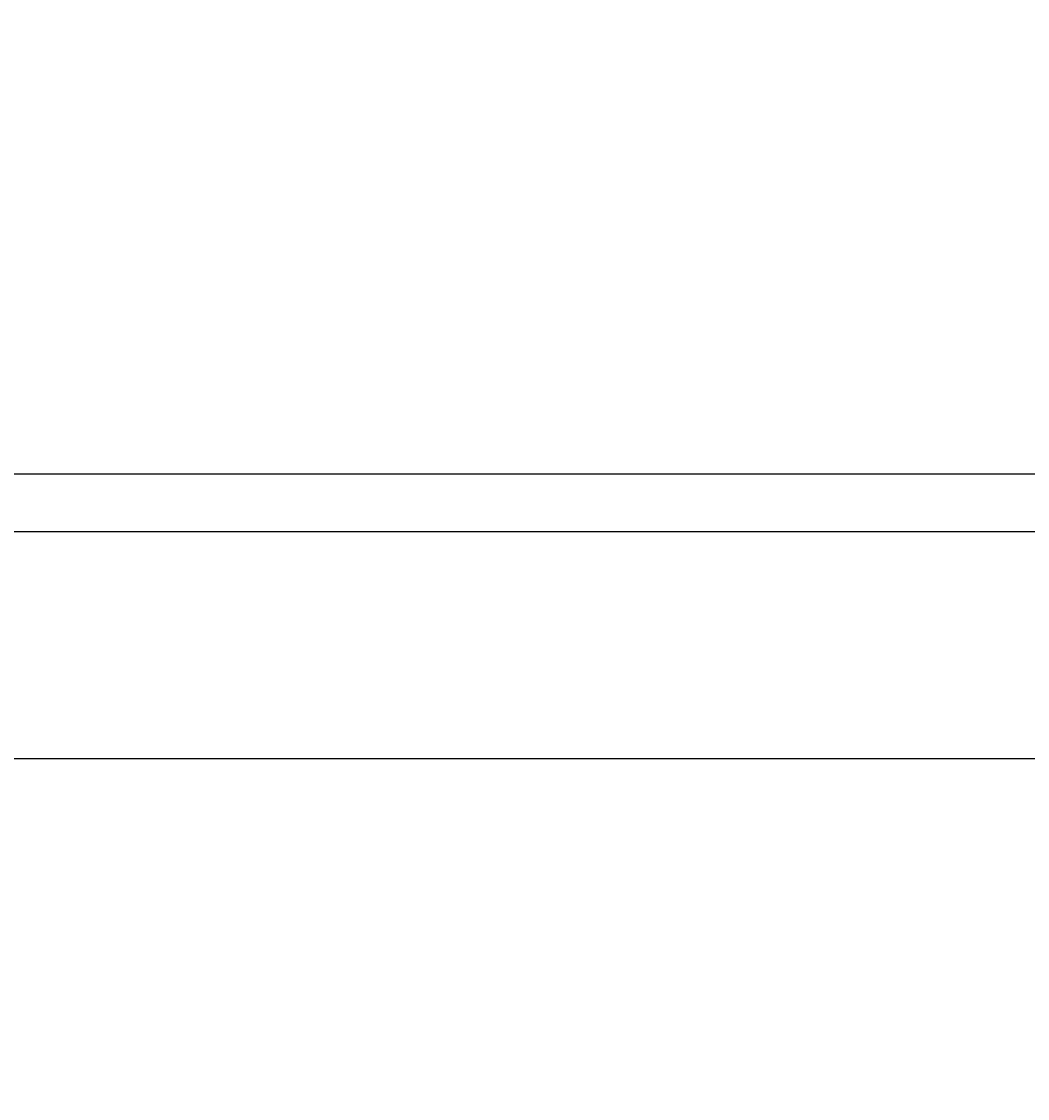
# Model space of a CAD drawing. Units: inches. Extents: x 1998 to 2588, y 1139 to 1977.
# Tile 96 of 134: x 2370 to 2397, y 1580 to 1608. Entities that reach past the tile are written whole.
import ezdxf

# ---------------------------------------------------------------- set-up
doc = ezdxf.new("R2010")
doc.units = ezdxf.units.IN
doc.layers.add('A-ANNO-DIMS', color=2, linetype='Continuous', lineweight=18)
doc.styles.get("Standard").update_dxf_attribs({"font": 'arial.ttf'})
doc.dimstyles.get("Standard").update_dxf_attribs({"dimtxt": 0.18, "dimasz": 0.18, "dimexe": 0.18, "dimexo": 0.0625, "dimgap": 0.09, "dimtad": 0, "dimtih": 1, "dimtoh": 1, "dimdec": 4, "dimzin": 0, "dimdsep": 46, "dimtxsty": 'Standard', "dimcen": 0.09, "dimadec": 0, "dimazin": 0, "dimtfac": 1, "dimtdec": 4, "dimtofl": 0, "dimtmove": 0, "dimatfit": 3, "dimfxl": 1, "dimtolj": 1, "dimtzin": 0, "dimarcsym": 0})

# ---------------------------------------------------------------- blocks, each defined once
blk = doc.blocks.new('*D30')
at = {"layer": 'A-ANNO-DIMS', "color": 0, "lineweight": -2, "transparency": 16777216}
for p, q in [((2407.91, 1636.732), (1997.843, 1636.732)), ((1998.023, 1636.552), (1998.023, 1615.913)), ((1998.023, 1594.912), (1998.023, 1615.552)), ((2407.91, 1594.732), (1997.843, 1594.732))]:
    blk.add_line(p, q, dxfattribs=at)
at = {"layer": 'A-ANNO-DIMS', "color": 0, "transparency": 16777216}
for points in [[(1997.993, 1636.552), (1998.053, 1636.552), (1998.023, 1636.732)], [(1997.993, 1594.912), (1998.053, 1594.912), (1998.023, 1594.732)]]:
    blk.add_solid(points, dxfattribs=at)
at = {"layer": 'Defpoints', "color": 0, "transparency": 16777216}
for p in [(1998.023, 1636.732), (2407.973, 1636.732), (2407.973, 1594.732)]:
    blk.add_point(p, dxfattribs=at)
at = {"layer": 'A-ANNO-DIMS', "color": 0, "transparency": 16777216, "insert": (1998.023, 1615.732), "char_height": 0.18, "attachment_point": 5}
blk.add_mtext('\\A1;42', dxfattribs=at)
blk = doc.blocks.new('*D34')
at = {"layer": 'A-ANNO-DIMS', "color": 0, "lineweight": -2, "transparency": 16777216}
for p, q in [((2407.91, 1594.732), (1997.843, 1594.732)), ((1998.023, 1594.552), (1998.023, 1558.913)), ((1998.023, 1522.912), (1998.023, 1558.552)), ((2407.91, 1522.732), (1997.843, 1522.732))]:
    blk.add_line(p, q, dxfattribs=at)
at = {"layer": 'A-ANNO-DIMS', "color": 0, "transparency": 16777216}
for points in [[(1997.993, 1594.552), (1998.053, 1594.552), (1998.023, 1594.732)], [(1997.993, 1522.912), (1998.053, 1522.912), (1998.023, 1522.732)]]:
    blk.add_solid(points, dxfattribs=at)
at = {"layer": 'Defpoints', "color": 0, "transparency": 16777216}
for p in [(1998.023, 1594.732), (2407.973, 1594.732), (2407.973, 1522.732)]:
    blk.add_point(p, dxfattribs=at)
at = {"layer": 'A-ANNO-DIMS', "color": 0, "transparency": 16777216, "insert": (1998.023, 1558.732), "char_height": 0.18, "attachment_point": 5}
blk.add_mtext('\\A1;72', dxfattribs=at)
blk = doc.blocks.new('*D39')
at = {"layer": 'A-ANNO-DIMS', "color": 0, "lineweight": -2, "transparency": 16777216}
for p, q in [((2115.035, 1628.742), (2588.309, 1628.742)), ((2588.129, 1628.562), (2588.129, 1612.685)), ((2588.129, 1596.444), (2588.129, 1612.321)), ((2115.035, 1596.264), (2588.309, 1596.264))]:
    blk.add_line(p, q, dxfattribs=at)
at = {"layer": 'A-ANNO-DIMS', "color": 0, "transparency": 16777216}
for points in [[(2588.099, 1628.562), (2588.159, 1628.562), (2588.129, 1628.742)], [(2588.099, 1596.444), (2588.159, 1596.444), (2588.129, 1596.264)]]:
    blk.add_solid(points, dxfattribs=at)
at = {"layer": 'Defpoints', "color": 0, "transparency": 16777216}
for p in [(2114.973, 1628.742), (2588.129, 1628.742), (2114.973, 1596.264)]:
    blk.add_point(p, dxfattribs=at)
at = {"layer": 'A-ANNO-DIMS', "color": 0, "transparency": 16777216, "insert": (2588.129, 1612.503), "char_height": 0.18, "attachment_point": 5}
blk.add_mtext('\\A1;32.48', dxfattribs=at)
blk = doc.blocks.new('*D42')
at = {"layer": 'A-ANNO-DIMS', "color": 0, "lineweight": -2, "transparency": 16777216}
for p, q in [((2287.535, 1588.732), (2588.309, 1588.732)), ((2588.129, 1588.552), (2588.129, 1555.914)), ((2588.129, 1522.912), (2588.129, 1555.55)), ((2287.535, 1522.732), (2588.309, 1522.732))]:
    blk.add_line(p, q, dxfattribs=at)
at = {"layer": 'A-ANNO-DIMS', "color": 0, "transparency": 16777216}
for points in [[(2588.099, 1588.552), (2588.159, 1588.552), (2588.129, 1588.732)], [(2588.099, 1522.912), (2588.159, 1522.912), (2588.129, 1522.732)]]:
    blk.add_solid(points, dxfattribs=at)
at = {"layer": 'Defpoints', "color": 0, "transparency": 16777216}
for p in [(2287.473, 1588.732), (2588.129, 1588.732), (2287.473, 1522.732)]:
    blk.add_point(p, dxfattribs=at)
at = {"layer": 'A-ANNO-DIMS', "color": 0, "transparency": 16777216, "insert": (2588.129, 1555.732), "char_height": 0.18, "attachment_point": 5}
blk.add_mtext('\\A1;66', dxfattribs=at)
blk = doc.blocks.new('*D43')
at = {"layer": 'A-ANNO-DIMS', "color": 0, "lineweight": -2, "transparency": 16777216}
for p, q in [((2407.973, 1594.67), (2407.973, 1138.602)), ((2345.973, 1588.67), (2345.973, 1138.602)), ((2346.153, 1138.782), (2376.754, 1138.782)), ((2407.793, 1138.782), (2377.191, 1138.782))]:
    blk.add_line(p, q, dxfattribs=at)
at = {"layer": 'A-ANNO-DIMS', "color": 0, "transparency": 16777216}
for points in [[(2346.153, 1138.812), (2346.153, 1138.752), (2345.973, 1138.782)], [(2407.793, 1138.812), (2407.793, 1138.752), (2407.973, 1138.782)]]:
    blk.add_solid(points, dxfattribs=at)
at = {"layer": 'Defpoints', "color": 0, "transparency": 16777216}
for p in [(2407.973, 1594.732), (2345.973, 1588.732), (2407.973, 1138.782)]:
    blk.add_point(p, dxfattribs=at)
at = {"layer": 'A-ANNO-DIMS', "color": 0, "transparency": 16777216, "insert": (2376.973, 1138.782), "char_height": 0.18, "attachment_point": 5}
blk.add_mtext('\\A1;62', dxfattribs=at)

msp = doc.modelspace()

# ---------------------------------------------------------------- dimensions: what is measured, and where the dimension line sits
at = {"layer": 'A-ANNO-DIMS'}
for base, p1, p2, override, picture, middle in [((1998.0229, 1636.7324), (2407.9729, 1594.7324), (2407.9729, 1636.7324), {"dimdec": 0, "dimlfac": 1, "dimrnd": 0, "dimzin": 0, "dimdsep": 46, "dimlunit": 2}, '*D30', (1998.0229, 1615.7324)), ((2588.1286, 1628.7416), (2114.9729, 1596.2642), (2114.9729, 1628.7416), {"dimdec": 2, "dimlfac": 1, "dimrnd": 0, "dimzin": 0, "dimdsep": 46, "dimlunit": 2}, '*D39', (2588.1286, 1612.5029)), ((1998.0229, 1594.7324), (2407.9729, 1522.7324), (2407.9729, 1594.7324), {"dimdec": 0, "dimlfac": 1, "dimrnd": 0, "dimzin": 0, "dimdsep": 46, "dimlunit": 2}, '*D34', (1998.0229, 1558.7324)), ((2588.1286, 1588.7324), (2287.4729, 1522.7324), (2287.4729, 1588.7324), {"dimdec": 0, "dimlfac": 1, "dimrnd": 0, "dimzin": 0, "dimdsep": 46, "dimlunit": 2}, '*D42', (2588.1286, 1555.7324))]:
    dim = msp.add_linear_dim(base=base, p1=p1, p2=p2, angle=90, dimstyle='Standard', override=override, dxfattribs=at)
    dim.commit()
    dim.dimension.update_dxf_attribs({"geometry": picture, "text_midpoint": middle})
dim = msp.add_linear_dim(base=(2407.9729, 1138.7824), p1=(2345.9729, 1588.7324), p2=(2407.9729, 1594.7324), dimstyle='Standard', override={"dimdec": 0, "dimlfac": 1, "dimrnd": 0, "dimzin": 0, "dimdsep": 46, "dimlunit": 2}, dxfattribs=at)
dim.commit()
dim.dimension.update_dxf_attribs({"geometry": '*D43', "text_midpoint": (2376.9729, 1138.7824)})

doc.saveas('drawing.dxf')
